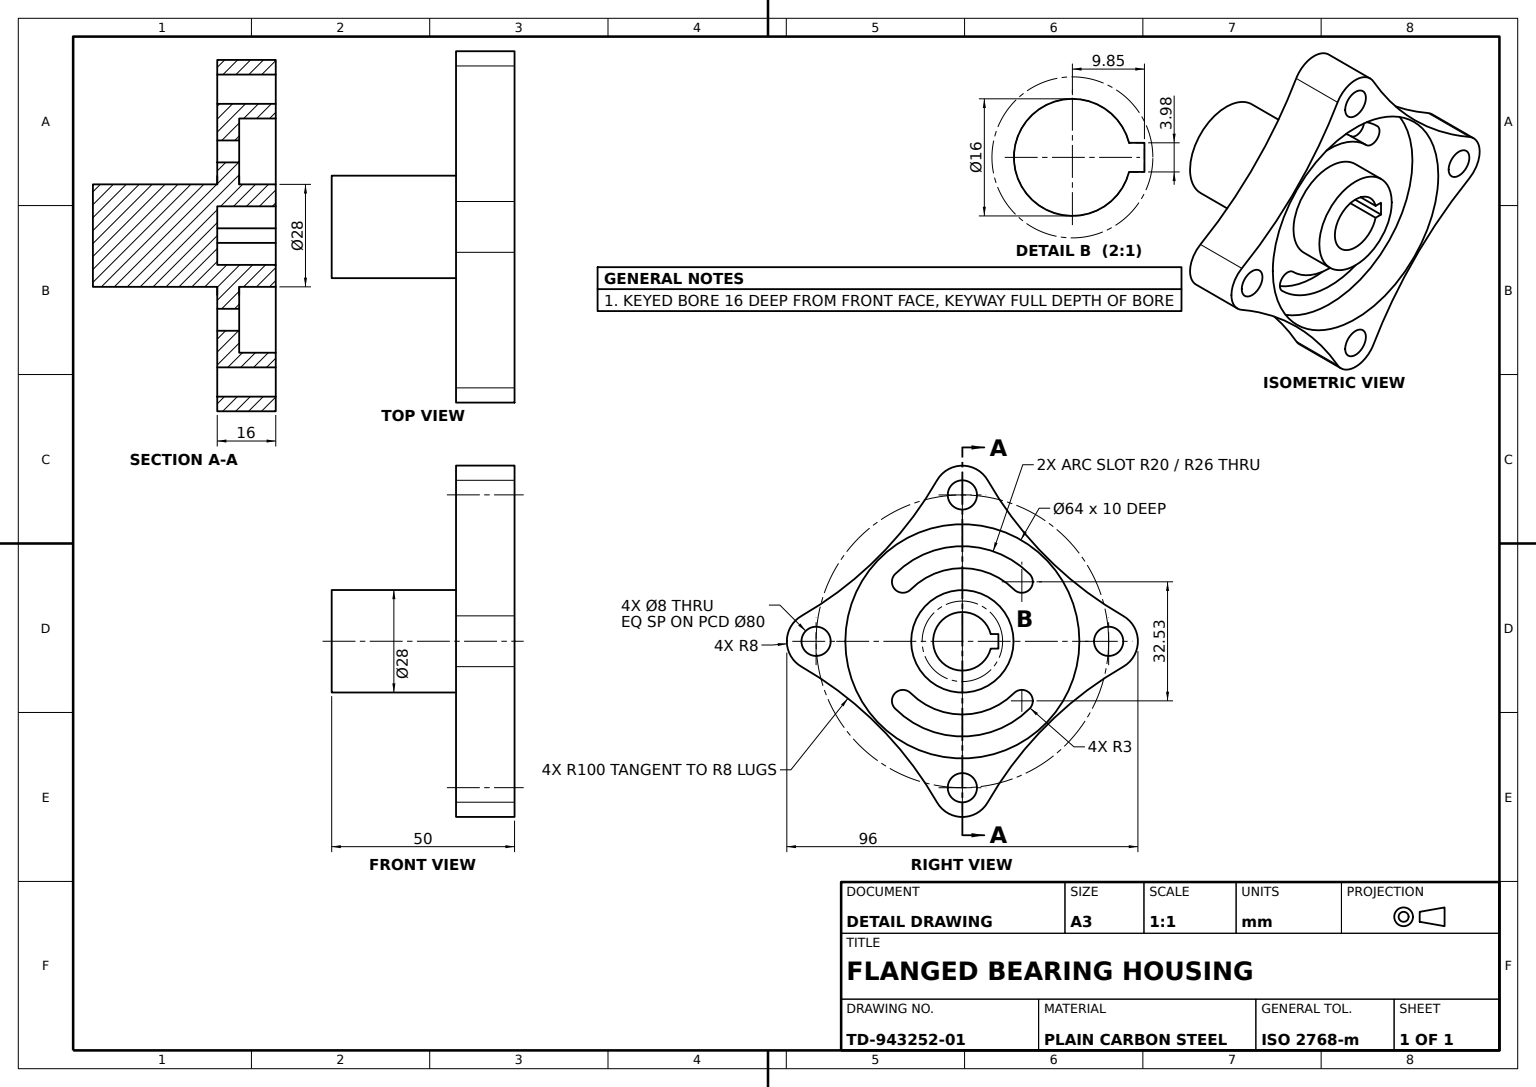
from build123d import *

# Parameters (mm, degrees)
FLANGE_PLATE_SKETCH_R    = 4
FLANGE_PLATE_SKETCH_R_2  = 32
FLANGE_PLATE_4_LUG_DEPTH = 16
FRONT_RECESS_32_SKETCH_R = 32
FRONT_RECESS_32_DEPTH    = 10
ARC_SLOTS_DEPTH          = 6
FRONT_HUB_14_SKETCH_R    = 14
FRONT_HUB_14_DEPTH       = 10
REAR_START               = 34
REAR_HUB_14_SKETCH_R     = 14
REAR_HUB_14_DEPTH        = 34
KEYED_BORE_8_DEPTH       = 16


with BuildPart() as part:
    # Flange Plate Sketch → Flange Plate 4-Lug (new body)
    # profile 1 of 2: a face of its own
    with BuildSketch(Plane.XY):
        with BuildLine():
            ThreePointArc((-6.940896525, -43.977933562), (-22.991424972, -22.991424972), (-43.977933562, -6.940896525))
            ThreePointArc((-43.977933562, -6.940896525), (-48, 0), (-43.977933562, 6.940896525))
            ThreePointArc((-43.977933562, 6.940896525), (-22.991424972, 22.991424972), (-6.940896525, 43.977933562))
            ThreePointArc((-6.940896525, 43.977933562), (0, 48), (6.940896525, 43.977933562))
            ThreePointArc((6.940896525, 43.977933562), (22.991424972, 22.991424972), (43.977933562, 6.940896525))
            ThreePointArc((43.977933562, 6.940896525), (48, 0), (43.977933562, -6.940896525))
            ThreePointArc((43.977933562, -6.940896525), (22.991424972, -22.991424972), (6.940896525, -43.977933562))
            ThreePointArc((6.940896525, -43.977933562), (0, -48), (-6.940896525, -43.977933562))
        make_face()
        with Locations((0, -40)):
            Circle(FLANGE_PLATE_SKETCH_R, mode=Mode.SUBTRACT)
        with Locations((-40, 0)):
            Circle(FLANGE_PLATE_SKETCH_R, mode=Mode.SUBTRACT)
        with Locations((40, 0)):
            Circle(FLANGE_PLATE_SKETCH_R, mode=Mode.SUBTRACT)
        with Locations((0, 40)):
            Circle(FLANGE_PLATE_SKETCH_R, mode=Mode.SUBTRACT)
        Circle(FLANGE_PLATE_SKETCH_R_2, mode=Mode.SUBTRACT)
    # profile 2 of 2: a face of its own
    with BuildSketch(Plane.XY):
        Circle(FLANGE_PLATE_SKETCH_R_2)
    extrude(amount=FLANGE_PLATE_4_LUG_DEPTH)

    # Front Recess Ø32 Sketch → Front Recess Ø32 (cut)
    with BuildSketch(Plane.XY.offset(16)):
        Circle(FRONT_RECESS_32_SKETCH_R)
    extrude(amount=-FRONT_RECESS_32_DEPTH, mode=Mode.SUBTRACT)

    # Arc Slots Sketch → Arc Slots (cut)
    with BuildSketch(Plane.XY.offset(6)):
        with BuildLine():
            ThreePointArc((-18.384776311, -18.384776311), (0, -26), (18.384776311, -18.384776311))
            ThreePointArc((18.384776311, -18.384776311), (18.384776311, -14.142135624), (14.142135624, -14.142135624))
            ThreePointArc((14.142135624, -14.142135624), (0, -20), (-14.142135624, -14.142135624))
            ThreePointArc((-14.142135624, -14.142135624), (-18.384776311, -14.142135624), (-18.384776311, -18.384776311))
        make_face()
        with BuildLine():
            ThreePointArc((14.142135624, 14.142135624), (0, 20), (-14.142135624, 14.142135624))
            ThreePointArc((-14.142135624, 14.142135624), (-18.384776311, 14.142135624), (-18.384776311, 18.384776311))
            ThreePointArc((-18.384776311, 18.384776311), (0, 26), (18.384776311, 18.384776311))
            ThreePointArc((18.384776311, 18.384776311), (18.384776311, 14.142135624), (14.142135624, 14.142135624))
        make_face()
    extrude(amount=-ARC_SLOTS_DEPTH, mode=Mode.SUBTRACT)

    # Front Hub Ø14 Sketch → Front Hub Ø14 (add)
    with BuildSketch(Plane.XY.offset(6)):
        Circle(FRONT_HUB_14_SKETCH_R)
    extrude(amount=FRONT_HUB_14_DEPTH)

    # Rear Hub Ø14 Sketch → Rear Hub Ø14 (add)
    with BuildSketch(Plane(origin=(0, 0, 0), x_dir=(-1, 0, 0), z_dir=(0, 0, -1)).offset(REAR_START)):
        with Locations(Location((0, 0, 0), (0, 0, 180))):
            Circle(REAR_HUB_14_SKETCH_R)
    extrude(amount=-REAR_HUB_14_DEPTH)

    # Keyed Bore Ø8 Sketch → Keyed Bore Ø8 (cut)
    with BuildSketch(Plane.XY.offset(16)):
        with BuildLine():
            Line((9.85, 0), (9.85, 1.99))
            Line((9.85, 1.99), (7.748541798, 1.99))
            ThreePointArc((7.748541798, 1.99), (-8, 0), (7.748541798, -1.99))
            Line((7.748541798, -1.99), (9.85, -1.99))
            Line((9.85, -1.99), (9.85, 0))
        make_face()
    extrude(amount=-KEYED_BORE_8_DEPTH, mode=Mode.SUBTRACT)


solid = part.part
